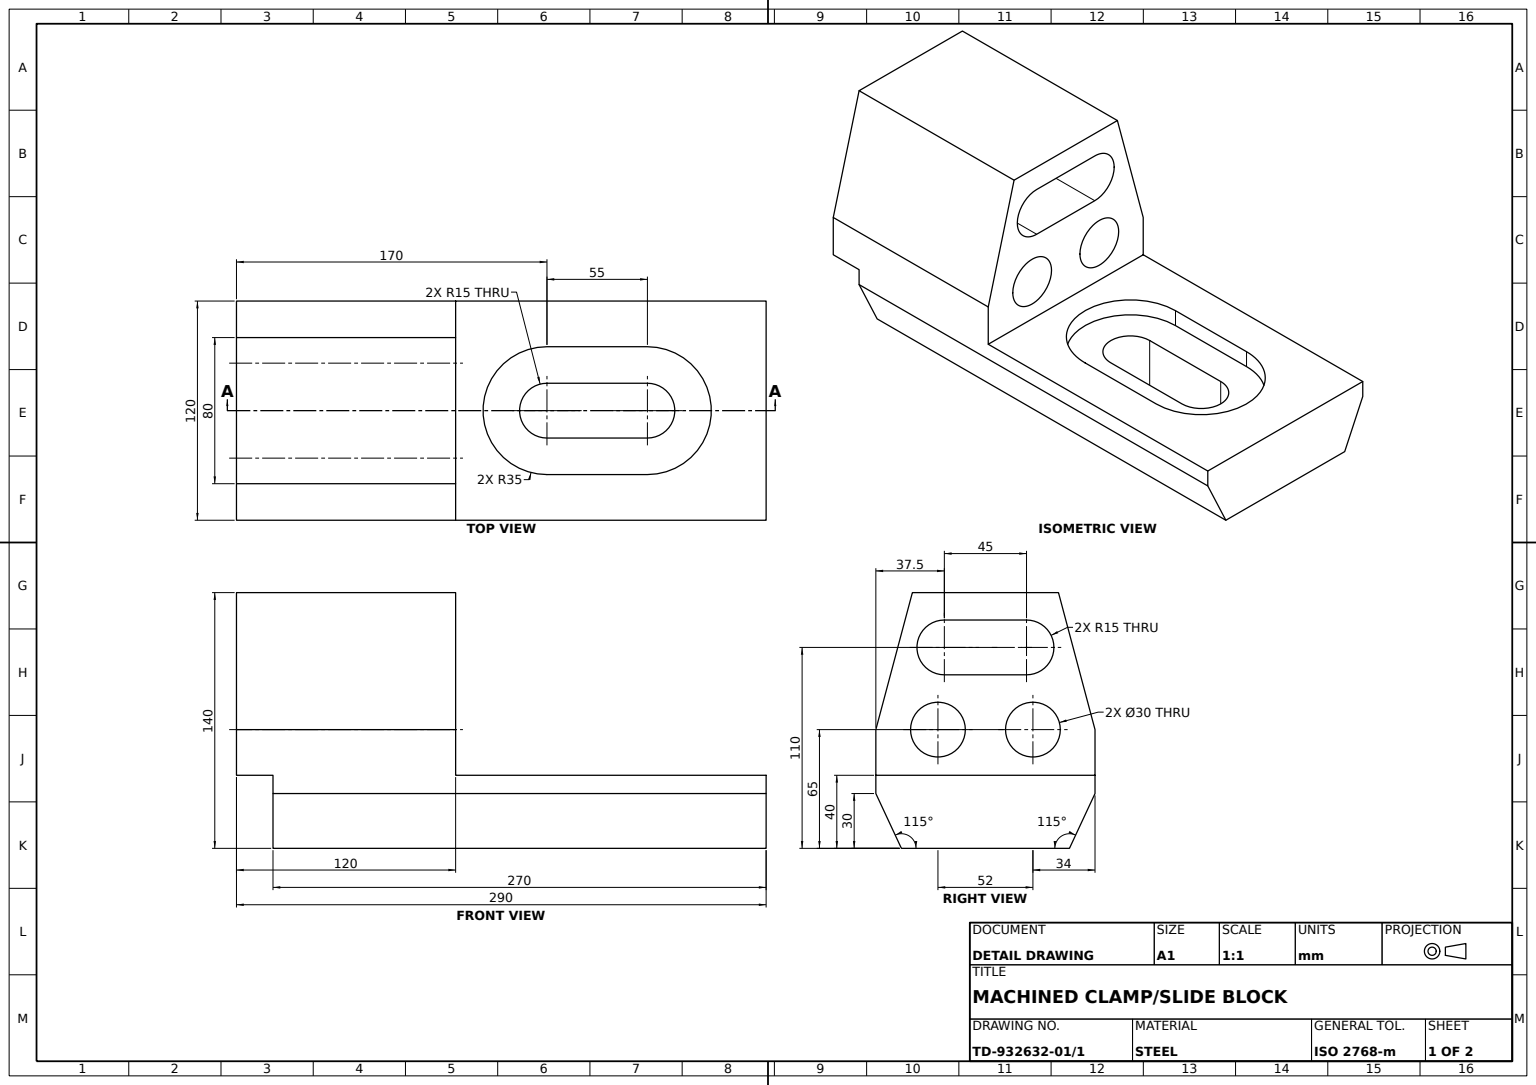
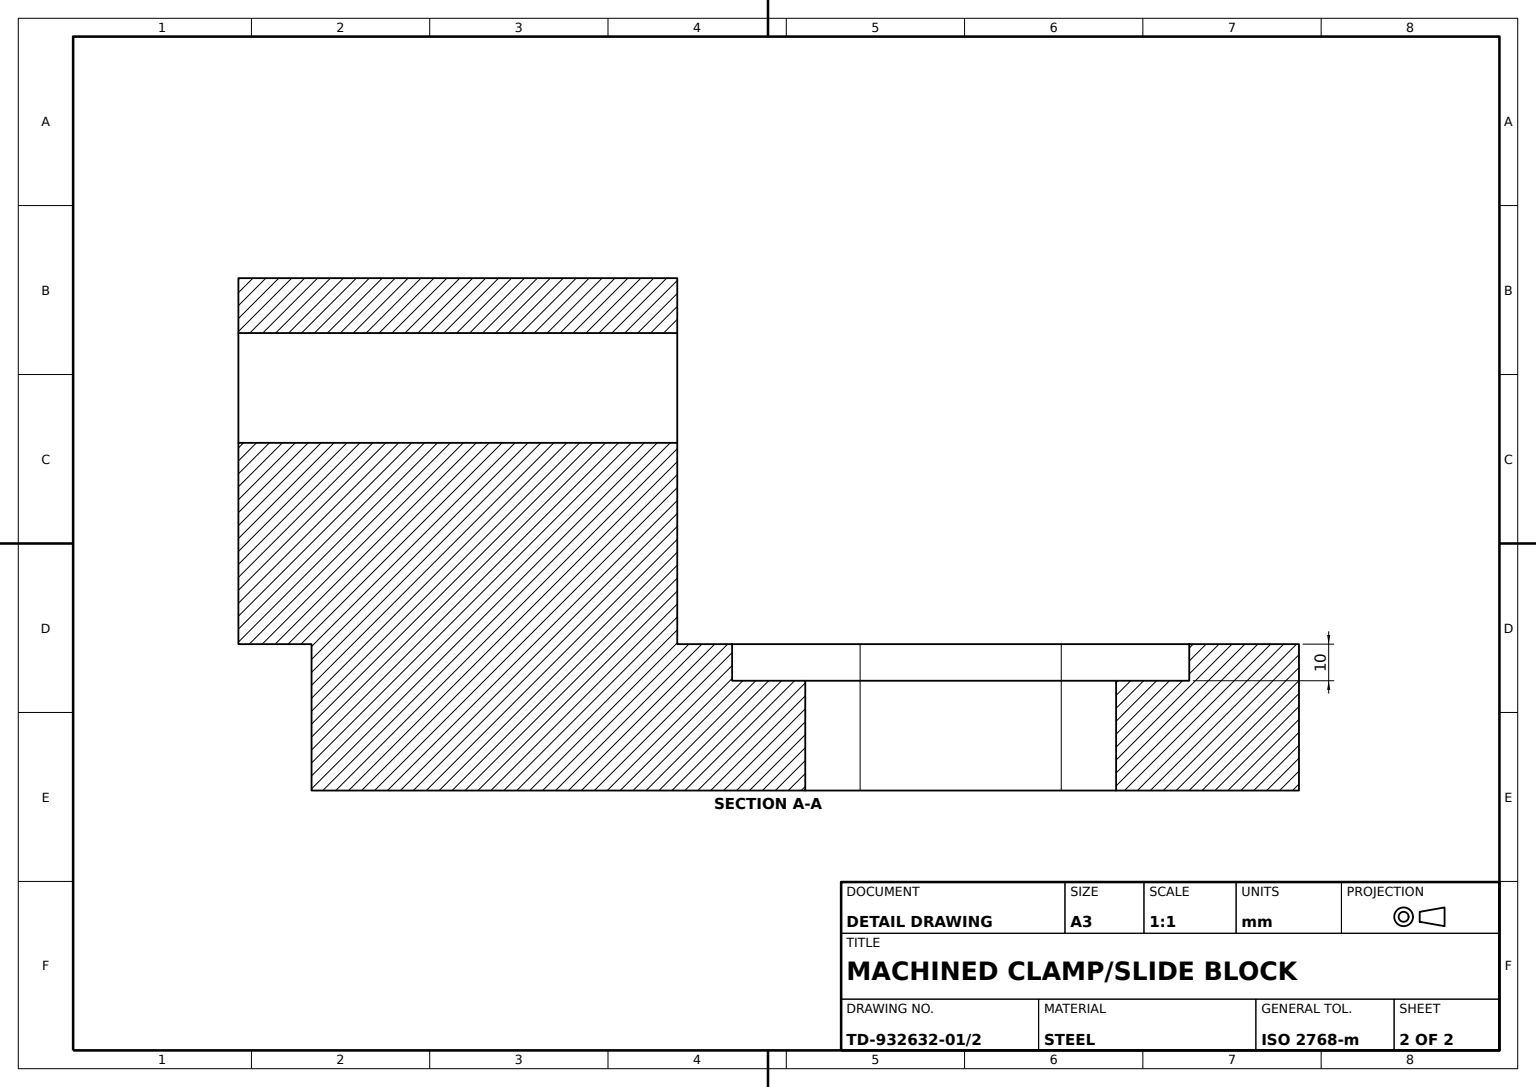
from build123d import *

# Parameters (mm, degrees)
WEDGE_BASE_RAIL_DEPTH         = 135
UPRIGHT_START                 = 20
UPRIGHT_BLOCK_DEPTH           = 120
BLOCK_SLOT_AND_HOLES_SKETCH_R = 15
BLOCK_SLOT_AND_HOLES_2X_DEPTH = 120
SLOT_COUNTERBORE_POCKET_DEPTH = 10
ADJUSTMENT_SLOT_THROUGH_DEPTH = 200.31131428


with BuildPart() as part:
    # Wedge Rail Profile Sketch → Wedge Base Rail (new, symmetric)
    with BuildSketch(Plane(origin=(0, 0, 0), x_dir=(0, 0, -1), z_dir=(1, 0, 0))):
        Polygon((-60, 0), (60, 0), (60, -10), (46.010770255, -40), (-46.010770255, -40), (-60, -10), align=None)
    extrude(amount=WEDGE_BASE_RAIL_DEPTH, both=True)

    # Upright Block Sketch → Upright Block (add)
    with BuildSketch(Plane.ZY.offset(135).offset(UPRIGHT_START)):
        Polygon((-60, 0), (-60, 25), (-40, 100), (40, 100), (60, 25), (60, 0), align=None)
    extrude(amount=-UPRIGHT_BLOCK_DEPTH)

    # Block Slot and Holes Sketch → Block Slot and Holes 2x (cut)
    with BuildSketch(Plane(origin=(-35, 0, 0), x_dir=(0, 0, -1), z_dir=(1, 0, 0))):
        with Locations((-26, 25)):
            Circle(BLOCK_SLOT_AND_HOLES_SKETCH_R)
        with Locations((26, 25)):
            Circle(BLOCK_SLOT_AND_HOLES_SKETCH_R)
        with BuildLine():
            Line((-22.5, 85), (22.5, 85))
            ThreePointArc((22.5, 85), (37.5, 70), (22.5, 55))
            Line((22.5, 55), (-22.5, 55))
            ThreePointArc((-22.5, 55), (-37.5, 70), (-22.5, 85))
        make_face()
    extrude(amount=-BLOCK_SLOT_AND_HOLES_2X_DEPTH, mode=Mode.SUBTRACT)

    # Slot Counterbore Sketch → Slot Counterbore Pocket (cut)
    with BuildSketch(Plane(origin=(0, 0, 0), x_dir=(1, 0, 0), z_dir=(0, 1, 0))):
        with BuildLine():
            Line((15, 35), (70, 35))
            ThreePointArc((70, 35), (105, 0), (70, -35))
            Line((70, -35), (15, -35))
            ThreePointArc((15, -35), (-20, 0), (15, 35))
        make_face()
    extrude(amount=-SLOT_COUNTERBORE_POCKET_DEPTH, mode=Mode.SUBTRACT)

    # Adjustment Slot Sketch → Adjustment Slot Through (cut, through all)
    with BuildSketch(Plane(origin=(0, -10, 0), x_dir=(1, 0, 0), z_dir=(0, 1, 0))):
        with BuildLine():
            Line((15, 15), (70, 15))
            ThreePointArc((70, 15), (85, 0), (70, -15))
            Line((70, -15), (15, -15))
            ThreePointArc((15, -15), (0, 0), (15, 15))
        make_face()
    extrude(amount=-ADJUSTMENT_SLOT_THROUGH_DEPTH, mode=Mode.SUBTRACT)


solid = part.part
